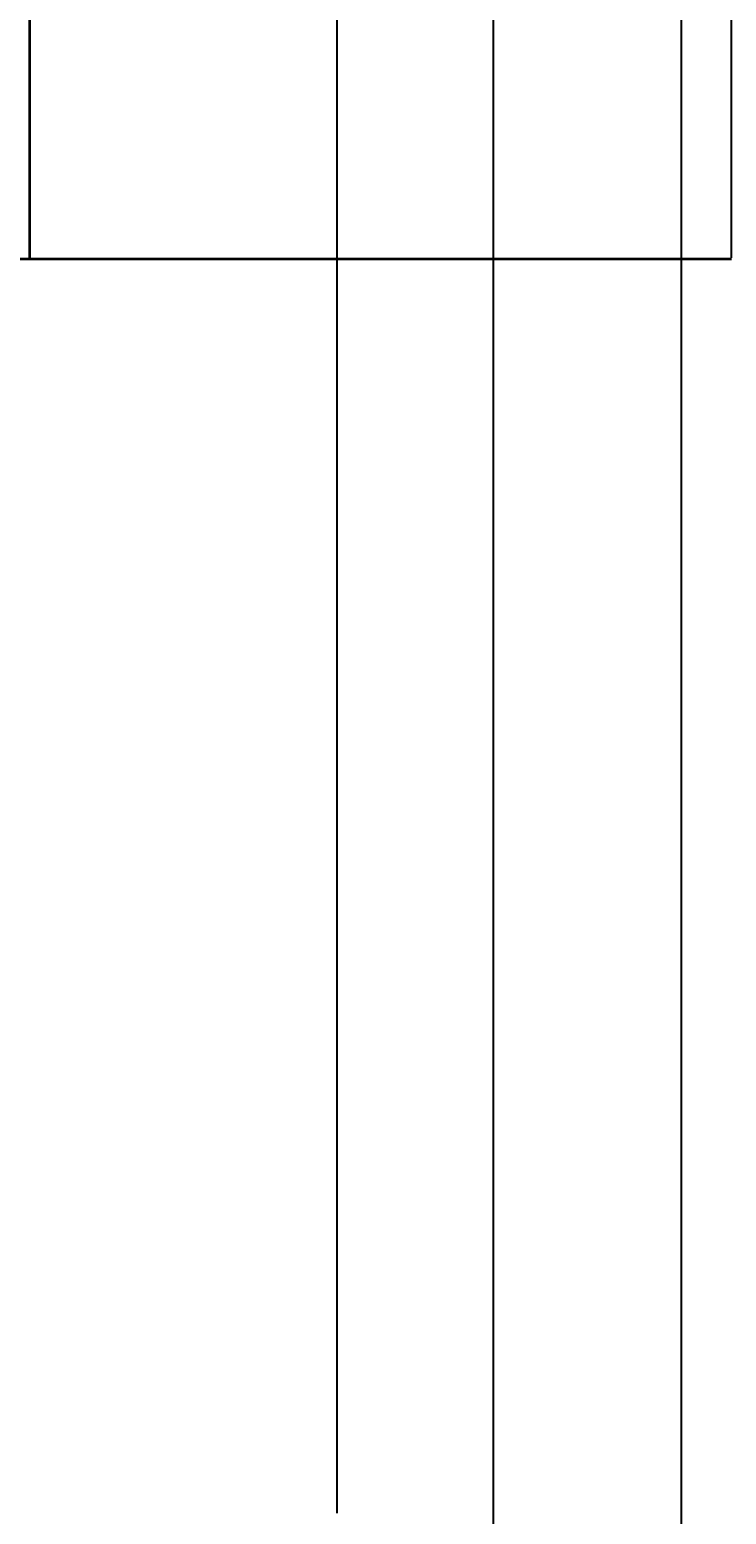
# Model space of a CAD drawing. Units: inches. Extents: x -26 to 776, y -22 to 650.
# Tile 33 of 62: x 192 to 231, y 420 to 504. Entities that reach past the tile are written whole.
import ezdxf

# ---------------------------------------------------------------- set-up
doc = ezdxf.new("R2010")
doc.units = ezdxf.units.IN
doc.header["$MEASUREMENT"] = 0
doc.layers.add('A-ANNO-DIMS', color=2, linetype='Continuous', lineweight=18)
doc.layers.add('A-WALL', color=7, linetype='Continuous', lineweight=35)
doc.styles.get("Standard").update_dxf_attribs({"font": 'arial.ttf'})
doc.dimstyles.get("Standard").update_dxf_attribs({"dimtxt": 0.5625, "dimasz": 0.18, "dimexe": 0.18, "dimexo": 0.0625, "dimgap": 0.09, "dimtad": 0, "dimtih": 1, "dimtoh": 1, "dimdec": 4, "dimzin": 0, "dimdsep": 46, "dimlunit": 4, "dimtxsty": 'Standard', "dimcen": 0.09, "dimadec": 0, "dimazin": 0, "dimtfac": 1, "dimtdec": 4, "dimtofl": 0, "dimtmove": 0, "dimatfit": 3, "dimfxl": 1, "dimtolj": 1, "dimtzin": 0, "dimarcsym": 0})

# ---------------------------------------------------------------- blocks, each defined once
blk = doc.blocks.new('*D15')
at = {"layer": 'A-ANNO-DIMS', "color": 0, "lineweight": -2, "transparency": 16777216}
for p, q in [((11.107, 491.489), (11.107, 649.856)), ((11.287, 649.676), (120.222, 649.676)), ((231.245, 649.676), (122.31, 649.676)), ((231.425, 491.489), (231.425, 649.856))]:
    blk.add_line(p, q, dxfattribs=at)
at = {"layer": 'A-ANNO-DIMS', "color": 0, "transparency": 16777216}
for points in [[(11.287, 649.706), (11.287, 649.646), (11.107, 649.676)], [(231.245, 649.706), (231.245, 649.646), (231.425, 649.676)]]:
    blk.add_solid(points, dxfattribs=at)
at = {"layer": 'Defpoints', "color": 0, "transparency": 16777216}
for p in [(231.425, 649.676), (11.107, 491.427), (231.425, 491.427)]:
    blk.add_point(p, dxfattribs=at)
at = {"layer": 'A-ANNO-DIMS', "color": 0, "transparency": 16777216, "insert": (121.266, 649.676), "char_height": 0.5625, "attachment_point": 5}
blk.add_mtext('\\A1;220.3', dxfattribs=at)
blk = doc.blocks.new('*D22')
at = {"layer": 'A-ANNO-DIMS', "color": 0, "lineweight": -2, "transparency": 16777216}
for p, q in [((22.889, 15.333), (22.889, 649.856)), ((23.069, 649.676), (119.19, 649.676)), ((217.773, 649.676), (121.652, 649.676)), ((217.953, 15.545), (217.953, 649.856))]:
    blk.add_line(p, q, dxfattribs=at)
at = {"layer": 'A-ANNO-DIMS', "color": 0, "transparency": 16777216}
for points in [[(23.069, 649.706), (23.069, 649.646), (22.889, 649.676)], [(217.773, 649.706), (217.773, 649.646), (217.953, 649.676)]]:
    blk.add_solid(points, dxfattribs=at)
at = {"layer": 'Defpoints', "color": 0, "transparency": 16777216}
for p in [(217.953, 649.676), (22.889, 15.27), (217.953, 15.482)]:
    blk.add_point(p, dxfattribs=at)
at = {"layer": 'A-ANNO-DIMS', "color": 0, "transparency": 16777216, "insert": (120.421, 649.676), "char_height": 0.5625, "attachment_point": 5}
blk.add_mtext('\\A1;195.06', dxfattribs=at)
blk = doc.blocks.new('*D34')
at = {"layer": 'A-ANNO-DIMS', "color": 0, "lineweight": -2, "transparency": 16777216}
for p, q in [((228.573, 528.296), (228.573, -21.315)), ((357.303, 528.361), (357.303, -21.315)), ((228.753, -21.135), (291.707, -21.135)), ((357.123, -21.135), (294.17, -21.135))]:
    blk.add_line(p, q, dxfattribs=at)
at = {"layer": 'A-ANNO-DIMS', "color": 0, "transparency": 16777216}
for points in [[(228.753, -21.105), (228.753, -21.165), (228.573, -21.135)], [(357.123, -21.105), (357.123, -21.165), (357.303, -21.135)]]:
    blk.add_solid(points, dxfattribs=at)
at = {"layer": 'Defpoints', "color": 0, "transparency": 16777216}
for p in [(357.303, 528.423), (228.573, 528.358), (357.303, -21.135)]:
    blk.add_point(p, dxfattribs=at)
at = {"layer": 'A-ANNO-DIMS', "color": 0, "transparency": 16777216, "insert": (292.938, -21.135), "char_height": 0.5625, "attachment_point": 5}
blk.add_mtext('\\A1;128.73', dxfattribs=at)
blk = doc.blocks.new('*D35')
at = {"layer": 'A-ANNO-DIMS', "color": 0, "lineweight": -2, "transparency": 16777216}
for p, q in [((82.134, 420.341), (82.134, 649.856)), ((82.314, 649.676), (144.382, 649.676)), ((208.911, 649.676), (146.843, 649.676)), ((209.091, 420.341), (209.091, 649.856))]:
    blk.add_line(p, q, dxfattribs=at)
at = {"layer": 'A-ANNO-DIMS', "color": 0, "transparency": 16777216}
for points in [[(82.314, 649.706), (82.314, 649.646), (82.134, 649.676)], [(208.911, 649.706), (208.911, 649.646), (209.091, 649.676)]]:
    blk.add_solid(points, dxfattribs=at)
at = {"layer": 'Defpoints', "color": 0, "transparency": 16777216}
for p in [(209.091, 649.676), (82.134, 420.278), (209.091, 420.278)]:
    blk.add_point(p, dxfattribs=at)
at = {"layer": 'A-ANNO-DIMS', "color": 0, "transparency": 16777216, "insert": (145.613, 649.676), "char_height": 0.5625, "attachment_point": 5}
blk.add_mtext('\\A1;126.96', dxfattribs=at)

msp = doc.modelspace()

# ---------------------------------------------------------------- linework, layer by layer
at = {"layer": 'A-WALL'}
for p, q in [((191.6782, 491.4269), (191.6782, 613.2713)), ((11.1074, 491.4269), (231.4249, 491.4269))]:
    msp.add_line(p, q, dxfattribs=at)

# ---------------------------------------------------------------- dimensions: what is measured, and where the dimension line sits
at = {"layer": 'A-ANNO-DIMS'}
for base, p1, p2, override, picture, middle in [((231.4249, 649.6763), (11.1074, 491.4269), (231.4249, 491.4269), {"dimdec": 1, "dimlfac": 1, "dimrnd": 0, "dimzin": 0, "dimdsep": 46, "dimlunit": 2}, '*D15', (121.2661, 649.6763)), ((217.9529, 649.6763), (22.8891, 15.2701), (217.9529, 15.4824), {"dimdec": 2, "dimlfac": 1, "dimrnd": 0, "dimzin": 0, "dimdsep": 46, "dimlunit": 2}, '*D22', (120.421, 649.6763)), ((209.091, 649.6763), (82.134, 420.2783), (209.091, 420.2783), {"dimdec": 2, "dimlfac": 1, "dimrnd": 0, "dimzin": 0, "dimdsep": 46, "dimlunit": 2}, '*D35', (145.6125, 649.6763)), ((357.3034, -21.1349), (228.5733, 528.3585), (357.3034, 528.4233), {"dimdec": 2, "dimlfac": 1, "dimrnd": 0, "dimzin": 0, "dimdsep": 46, "dimlunit": 2}, '*D34', (292.9384, -21.1349))]:
    dim = msp.add_linear_dim(base=base, p1=p1, p2=p2, dimstyle='Standard', override=override, dxfattribs=at)
    dim.commit()
    dim.dimension.update_dxf_attribs({"geometry": picture, "text_midpoint": middle})

doc.saveas('drawing.dxf')
